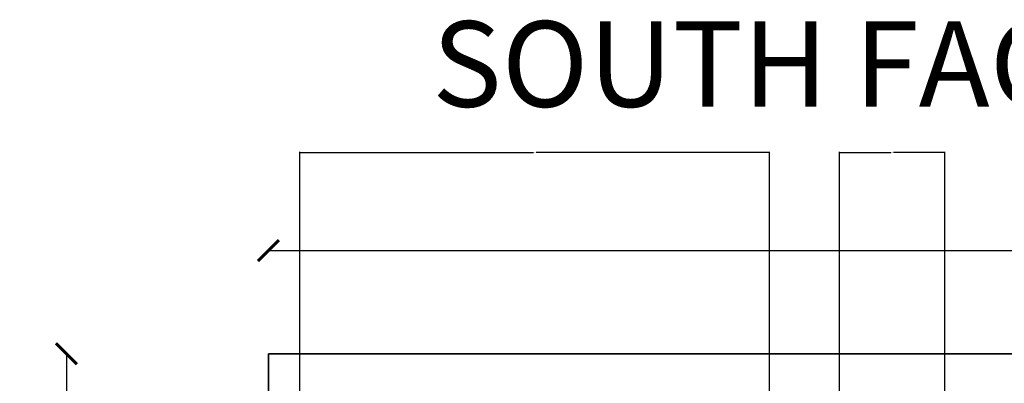
# Model space of a CAD drawing. Units: inches. Extents: x 318 to 927, y -1130 to 13.
# Tile 16 of 17: x 318 to 599, y -91 to 13. Entities that reach past the tile are written whole.
import ezdxf

# ---------------------------------------------------------------- set-up
doc = ezdxf.new("R2010")
doc.units = ezdxf.units.IN
doc.header["$MEASUREMENT"] = 0
for name, color, linetype, lineweight in [('A-ANNO-DIMS', 1, 'Continuous', 18), ('A-ANNO-TEXT', 8, 'Continuous', 25), ('wall', 1, 'Continuous', 35)]:
    doc.layers.add(name, color=color, linetype=linetype, lineweight=lineweight)
doc.styles.get("Standard").update_dxf_attribs({"font": 'arial.ttf'})
doc.dimstyles.get("Standard").update_dxf_attribs({"dimtxt": 0.18, "dimasz": 0.18, "dimexe": 0.18, "dimexo": 0.0625, "dimgap": 0.09, "dimtad": 0, "dimtih": 1, "dimtoh": 1, "dimdec": 1, "dimzin": 0, "dimdsep": 46, "dimlunit": 4, "dimtxsty": 'Standard', "dimcen": 0.09, "dimadec": 0, "dimazin": 0, "dimtfac": 1, "dimtdec": 1, "dimtofl": 0, "dimtmove": 0, "dimatfit": 3, "dimfxl": 1, "dimtolj": 1, "dimtzin": 0, "dimarcsym": 0})

# ---------------------------------------------------------------- blocks, each defined once
blk = doc.blocks.new('_ArchTick')
at = {"color": 0, "linetype": 'ByBlock', "const_width": 0.15}
blk.add_lwpolyline([(-0.5, -0.5), (0.5, 0.5)], dxfattribs=at)
blk = doc.blocks.new('*D3')
at = {"layer": 'A-ANNO-DIMS', "color": 0, "lineweight": -2, "transparency": 16777216}
blk.add_line((388.89, -53.46), (868.89, -53.46), dxfattribs=at)
at = {"layer": 'Defpoints', "color": 0, "transparency": 16777216}
for p in [(868.89, -53.46), (388.89, -82.91), (868.89, -82.91)]:
    blk.add_point(p, dxfattribs=at)
at = {"layer": 'A-ANNO-DIMS', "color": 0, "lineweight": -2, "transparency": 16777216, "xscale": 6, "yscale": 6, "zscale": 6, "rotation": 180}
blk.add_blockref('_ArchTick', (388.89, -53.46), dxfattribs=at)
at = {"layer": 'A-ANNO-DIMS', "color": 0, "lineweight": -2, "transparency": 16777216, "xscale": 6, "yscale": 6, "zscale": 6}
blk.add_blockref('_ArchTick', (868.89, -53.46), dxfattribs=at)
at = {"layer": 'A-ANNO-DIMS', "color": 0, "transparency": 16777216, "insert": (628.89, -45.37), "char_height": 8, "attachment_point": 5}
blk.add_mtext("\\A1;40'", dxfattribs=at)
blk = doc.blocks.new('*D4')
at = {"layer": 'A-ANNO-DIMS', "color": 0, "lineweight": -2, "transparency": 16777216}
blk.add_line((331.26, -82.91), (331.26, -1042.91), dxfattribs=at)
at = {"layer": 'Defpoints', "color": 0, "transparency": 16777216}
for p in [(388.89, -82.91), (331.26, -1042.91), (388.89, -1042.91)]:
    blk.add_point(p, dxfattribs=at)
at = {"layer": 'A-ANNO-DIMS', "color": 0, "lineweight": -2, "transparency": 16777216, "xscale": 6, "yscale": 6, "zscale": 6}
for p, rotation in [((331.26, -82.91), 90), ((331.26, -1042.91), 270)]:
    blk.add_blockref('_ArchTick', p, dxfattribs=dict(at, rotation=rotation))
at = {"layer": 'A-ANNO-DIMS', "color": 0, "transparency": 16777216, "insert": (323.18, -562.91), "char_height": 8, "attachment_point": 5, "rotation": 90}
blk.add_mtext("\\A1;80'", dxfattribs=at)
blk = doc.blocks.new('*D30')
at = {"layer": 'A-ANNO-DIMS', "color": 0, "lineweight": -2, "transparency": 16777216}
for p, q in [((551.89, -820.85), (551.89, -25.23)), ((581.89, -820.85), (581.89, -25.23)), ((552.07, -25.41), (566.56, -25.41)), ((581.71, -25.41), (567.23, -25.41))]:
    blk.add_line(p, q, dxfattribs=at)
at = {"layer": 'A-ANNO-DIMS', "color": 0, "transparency": 16777216}
for points in [[(552.07, -25.38), (552.07, -25.44), (551.89, -25.41)], [(581.71, -25.38), (581.71, -25.44), (581.89, -25.41)]]:
    blk.add_solid(points, dxfattribs=at)
at = {"layer": 'Defpoints', "color": 0, "transparency": 16777216}
for p in [(581.89, -25.41), (551.89, -820.91), (581.89, -820.91)]:
    blk.add_point(p, dxfattribs=at)
at = {"layer": 'A-ANNO-DIMS', "color": 0, "transparency": 16777216, "insert": (566.89, -25.41), "char_height": 0.18, "attachment_point": 5}
blk.add_mtext('\\A1;2\'-6"', dxfattribs=at)
blk = doc.blocks.new('*D33')
at = {"layer": 'A-ANNO-DIMS', "color": 0, "lineweight": -2, "transparency": 16777216}
for p, q in [((397.89, -370.85), (397.89, -25.23)), ((531.89, -370.85), (531.89, -25.23)), ((398.07, -25.41), (464.5, -25.41)), ((531.71, -25.41), (465.28, -25.41))]:
    blk.add_line(p, q, dxfattribs=at)
at = {"layer": 'A-ANNO-DIMS', "color": 0, "transparency": 16777216}
for points in [[(398.07, -25.38), (398.07, -25.44), (397.89, -25.41)], [(531.71, -25.38), (531.71, -25.44), (531.89, -25.41)]]:
    blk.add_solid(points, dxfattribs=at)
at = {"layer": 'Defpoints', "color": 0, "transparency": 16777216}
for p in [(531.89, -25.41), (397.89, -370.91), (531.89, -370.91)]:
    blk.add_point(p, dxfattribs=at)
at = {"layer": 'A-ANNO-DIMS', "color": 0, "transparency": 16777216, "insert": (464.89, -25.41), "char_height": 0.18, "attachment_point": 5}
blk.add_mtext('\\A1;11\'-2"', dxfattribs=at)

msp = doc.modelspace()

# ---------------------------------------------------------------- linework, layer by layer
at = {"layer": 'wall'}
for p, q in [((388.89, -82.91), (388.89, -1042.91)), ((868.89, -82.91), (388.89, -82.91))]:
    msp.add_line(p, q, dxfattribs=at)

# ---------------------------------------------------------------- texts
at = {"layer": 'A-ANNO-TEXT', "insert": (435.61, 12.07), "char_height": 24.4528, "attachment_point": 1}
msp.add_mtext_dynamic_manual_height_columns('SOUTH FACING HOUSE', width=395.3147, gutter_width=4.08, heights=[0], dxfattribs=at)

# ---------------------------------------------------------------- dimensions: what is measured, and where the dimension line sits
at = {"layer": 'A-ANNO-DIMS'}
for base, p1, p2, override, picture, middle in [((531.89, -25.41), (397.89, -370.91), (531.89, -370.91), {"dimdec": 1, "dimlfac": 1, "dimrnd": 0, "dimzin": 1, "dimdsep": 46, "dimlunit": 4, "dimfrac": 2}, '*D33', (464.89, -25.41)), ((581.89, -25.41), (551.89, -820.91), (581.89, -820.91), {"dimdec": 1, "dimlfac": 1, "dimrnd": 0, "dimzin": 1, "dimdsep": 46, "dimlunit": 4, "dimfrac": 2}, '*D30', (566.89, -25.41)), ((868.89, -53.46), (388.89, -82.91), (868.89, -82.91), {"dimtxt": 8, "dimasz": 6, "dimgap": 4, "dimtad": 1, "dimblk1": 'ArchTick', "dimblk2": 'ArchTick', "dimsah": 1, "dimse1": 1, "dimse2": 1, "dimclrd": 0, "dimclre": 0, "dimclrt": 0}, '*D3', (628.89, -45.37))]:
    dim = msp.add_linear_dim(base=base, p1=p1, p2=p2, dimstyle='Standard', override=override, dxfattribs=at)
    dim.commit()
    dim.dimension.update_dxf_attribs({"geometry": picture, "text_midpoint": middle})
dim = msp.add_linear_dim(base=(331.26, -1042.91), p1=(388.89, -82.91), p2=(388.89, -1042.91), angle=90, dimstyle='Standard', override={"dimtxt": 8, "dimasz": 6, "dimgap": 4, "dimtad": 1, "dimtih": 0, "dimblk1": 'ArchTick', "dimblk2": 'ArchTick', "dimsah": 1, "dimse1": 1, "dimse2": 1, "dimclrd": 0, "dimclre": 0, "dimclrt": 0}, dxfattribs=at)
dim.commit()
dim.dimension.update_dxf_attribs({"geometry": '*D4', "text_midpoint": (323.18, -562.91)})

doc.saveas('drawing.dxf')
